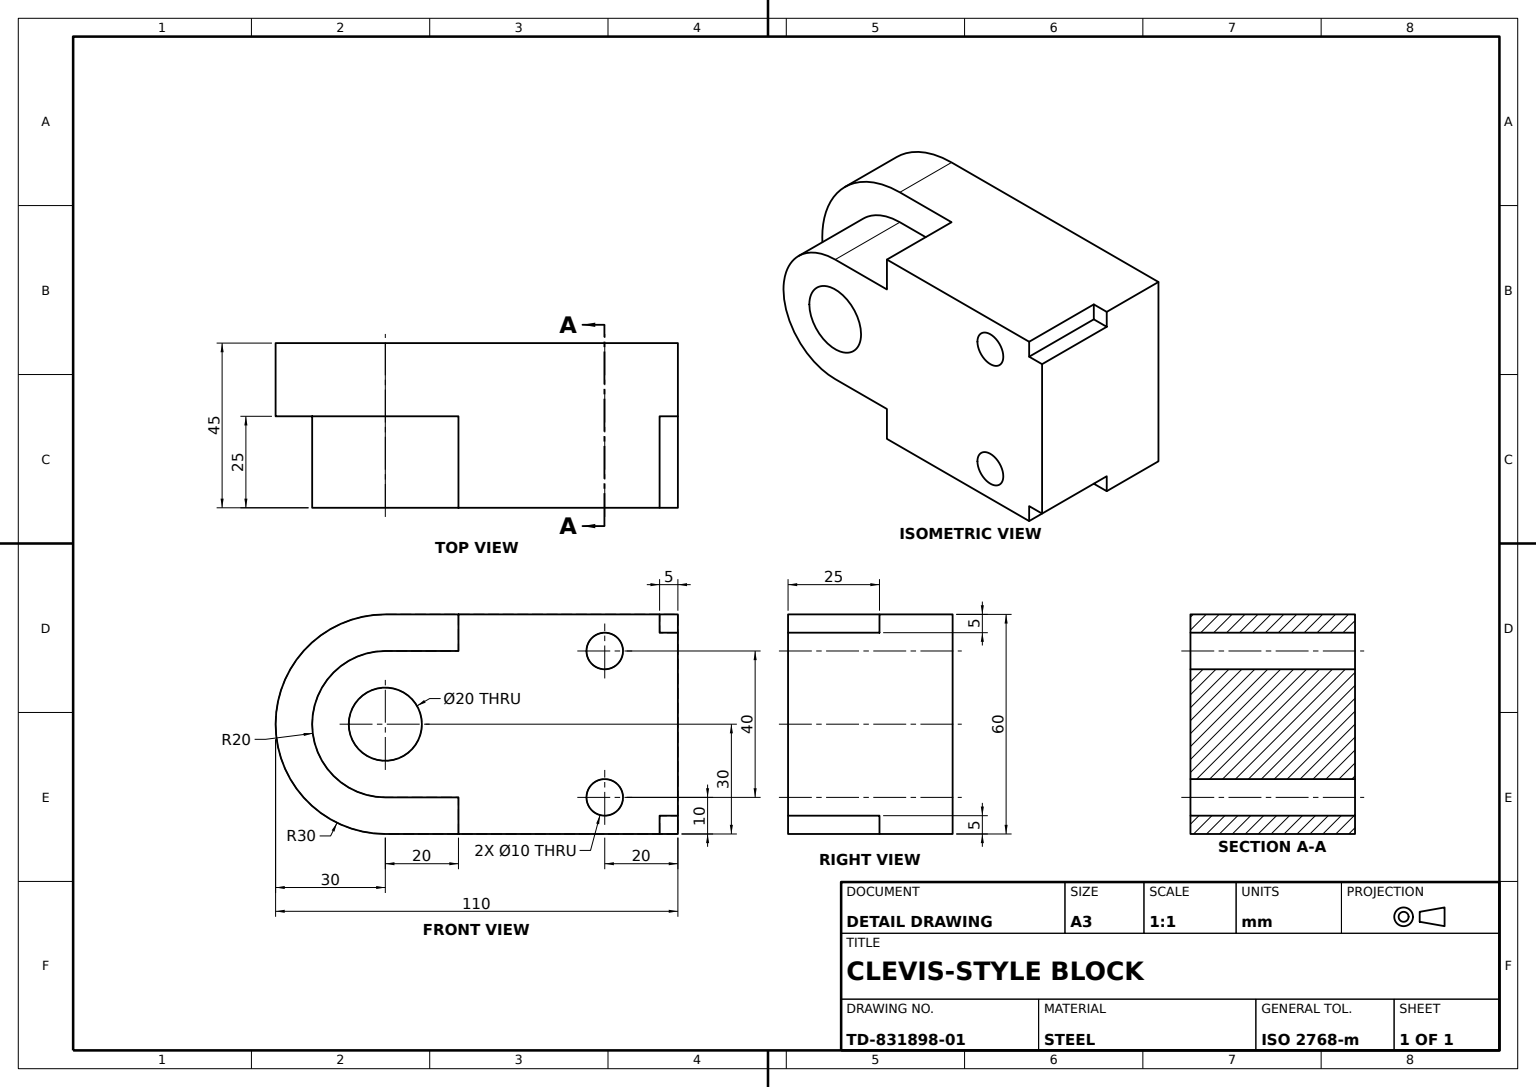
SolidWorks part; units mm, degrees
material "Plain Carbon Steel"
ref_plane "Front Plane" through (0, 0, 0) normal (0, 0, 1) x (1, 0, 0)
ref_plane "Top Plane" through (0, 0, 0) normal (0, 1, 0) x (1, 0, 0)
ref_plane "Right Plane" through (0, 0, 0) normal (1, 0, 0) x (0, 0, -1)
sketch "Base Block Sketch" plane through (0, 0, 0) normal (0, 0, 1) x (1, 0, 0)
  line L0 (0, 30) -> (80, 30)
  line L5 (80, 30) -> (80, -30)
  line L6 (80, -30) -> (0, -30)
  arc A0 (0, 30) -> (0, -30) centre (0, 0) ccw
  circle A1 centre (0, 0) radius 10
  dimension "D1" = 60
  dimension "D3" = 20
  dimension "D2" = 80
extrude "Base Block" add sketch "Base Block Sketch" along normal blind 20
sketch "Lug Boss Sketch" plane through (0, 0, 20) normal (0, 0, 1) x (1, 0, 0)
  line L0 (0, 20) -> (20, 20)
  line L1 (20, 20) -> (20, 30)
  line L2 (80, 30) -> (0, 30) construction
  line L3 (20, 30) -> (75, 30)
  line L4 (80, 25) -> (80, -25)
  line L5 (75, -30) -> (20, -30)
  line L6 (0, -30) -> (80, -30) construction
  line L7 (20, -30) -> (20, -20)
  line L8 (20, -20) -> (0, -20)
  line L12 (80, 25) -> (75, 25)
  line L13 (75, 30) -> (75, 25)
  line L16 (80, -25) -> (75, -25)
  line L17 (75, -30) -> (75, -25)
  circle A0 centre (0, 0) radius 10
  arc A1 (0, 20) -> (0, -20) centre (0, 0) ccw
  circle A2 centre (60, 20) radius 5
  circle A3 centre (60, -20) radius 5
  dimension "D1" = 20
  dimension "D2" = 40
  dimension "D3" = 10
  dimension "D4" = 10
  dimension "D5" = 60
  dimension "D6" = 80
  dimension "D7" = 10
  dimension "D8" = 10
  dimension "D9" = 5
extrude "Lug Boss With Holes" add sketch "Lug Boss Sketch" along normal blind 25
sketch "Slot Cut Sketch" plane through (0, 0, 45) normal (0, 0, 1) x (1, 0, 0)
  circle A0 centre (60, -20) radius 5 construction
  circle A1 centre (60, 20) radius 5 construction
  circle A2 centre (60, -20) radius 5
  circle A3 centre (60, 20) radius 5
extrude "Slot Cut" cut sketch "Slot Cut Sketch" against normal through all
